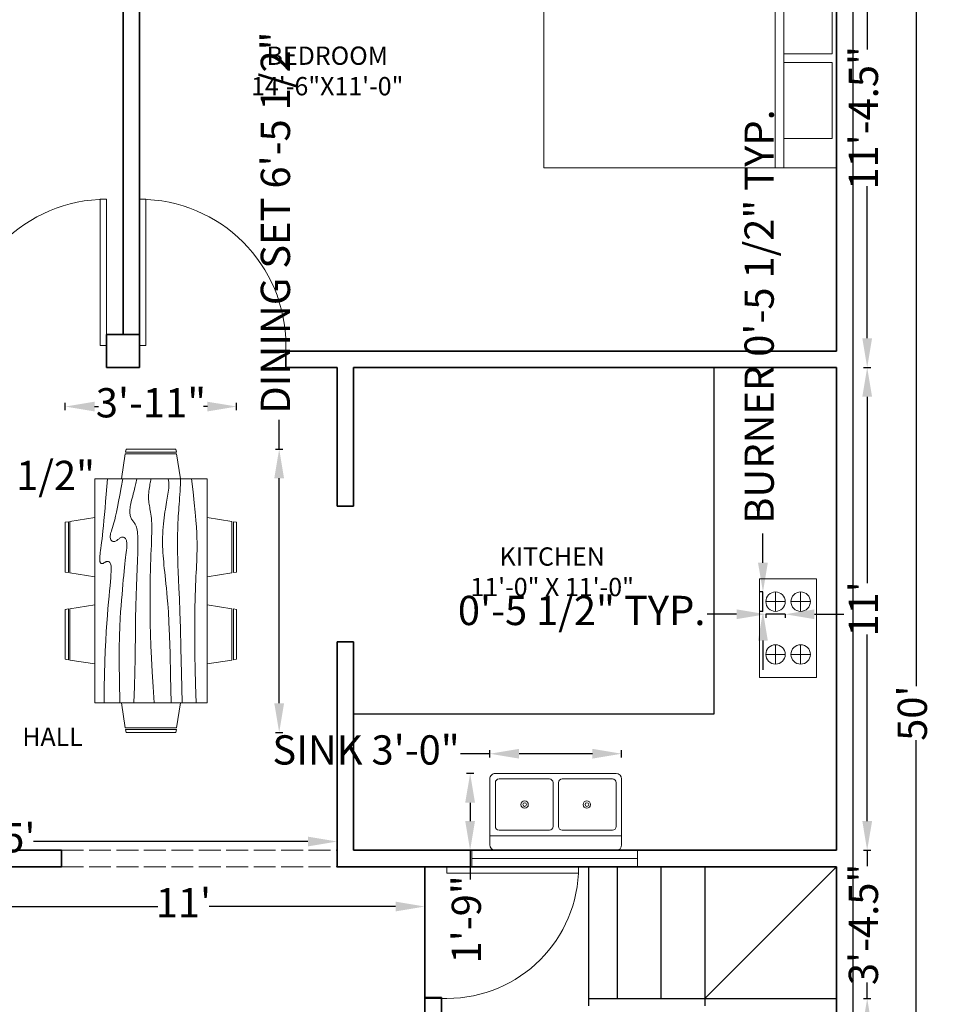
# Model space of a CAD drawing. Units: inches. Extents: x 2174 to 2692, y 577 to 1264.
# Tile 4 of 5: x 2442 to 2692, y 841 to 1110. Entities that reach past the tile are written whole.
import ezdxf

# ---------------------------------------------------------------- set-up
doc = ezdxf.new("R2010")
doc.units = ezdxf.units.IN
doc.linetypes.add('ACAD_ISO02W100', pattern=[15, 12, -3])
for name, color, linetype, lineweight in [('A-ANNO-DIMS', 2, 'Continuous', 13), ('A-AREA-IDEN', 7, 'Continuous', 18), ('A-COLS', 7, 'Continuous', 35), ('A-DOOR', 3, 'Continuous', 18), ('A-EQPM', 8, 'Continuous', 18), ('A-FLOR-CASE', 8, 'Continuous', 25), ('A-FLOR-FIXT', 9, 'Continuous', 18), ('A-FLOR-STRS', 7, 'Continuous', 25), ('A-FURN', 8, 'Continuous', 18), ('A-GLAZ', 4, 'Continuous', 18), ('A-WALL', 7, 'Continuous', 35), ('A-WALL-OVHD', 8, 'ACAD_ISO02W100', 18), ('C-PROP', 7, 'Continuous', 25)]:
    doc.layers.add(name, color=color, linetype=linetype, lineweight=lineweight)
doc.styles.get("Standard").update_dxf_attribs({"font": 'arial.ttf'})
doc.dimstyles.new('ISO-25', dxfattribs={"dimtxt": 8, "dimasz": 8, "dimexe": 1, "dimexo": 1, "dimtad": 0, "dimdec": 1, "dimlunit": 3, "dimtxsty": 'Standard', "dimcen": 2.5, "dimclrd": 1, "dimclre": 1, "dimclrt": 1, "dimadec": 0, "dimazin": 0, "dimtfac": 1, "dimtdec": 1, "dimtmove": 0, "dimatfit": 3, "dimfxl": 1, "dimfxlon": 1, "dimarcsym": 0})

# ---------------------------------------------------------------- blocks, each defined once
blk = doc.blocks.new('Dining Set - 36 x 72 in.')
for p, q in [((-22.2343, 26.00059), (-23.4847, 17.99762)), ((-22.2304, 26), (-5.7608, 26)), ((-22, 27.5), (-22.1562, 26.50042)), ((-5.8416, 26.5), (-22.1534, 26.5)), ((-22, 27.5), (-6, 27.5)), ((-5.8437, 26.49966), (-6, 27.5)), ((-4.5152, 17.99762), (-5.7655, 25.99926)), ((5.7657, 26.00059), (4.5153, 17.99762)), ((5.7696, 26), (22.2392, 26)), ((6, 27.5), (5.8438, 26.50042)), ((22.1584, 26.5), (5.8466, 26.5)), ((6, 27.5), (22, 27.5)), ((22.1563, 26.49966), (22, 27.5)), ((23.4848, 17.99762), (22.2345, 25.99926)), ((36, 18), (-36, 18)), ((-36, 18), (-36, -18)), ((36, -18), (36, 18)), ((-44.0006, 8.23428), (-35.9976, 9.48474)), ((44.0006, 8.23428), (35.9976, 9.48474)), ((-45.5, 8), (-44.5004, 8.15617)), ((-45.5, 8), (-45.5, -8)), ((-44.5, -8.15843), (-44.5, 8.15338)), ((-44, 8.23041), (-44, -8.23915)), ((44, 8.23041), (44, -8.23915)), ((44.5, -8.15843), (44.5, 8.15338)), ((45.5, 8), (44.5005, 8.15617)), ((45.5, 8), (45.5, -8)), ((-44.4997, -8.15631), (-45.5, -8)), ((-35.9976, -9.48476), (-43.9993, -8.2345)), ((35.9976, -9.48476), (43.9993, -8.2345)), ((44.4997, -8.15631), (45.5, -8)), ((-36, -18), (36, -18)), ((-22.2343, -26.0006), (-23.4847, -17.99762)), ((-4.5152, -17.99762), (-5.7655, -25.99928)), ((5.7657, -26.0006), (4.5153, -17.99762)), ((23.4848, -17.99762), (22.2345, -25.99928)), ((-22.2304, -26), (-5.7608, -26)), ((-22, -27.5), (-22.1562, -26.50044)), ((-5.8416, -26.5), (-22.1534, -26.5)), ((-22, -27.5), (-6, -27.5)), ((-5.8437, -26.49967), (-6, -27.5)), ((5.7696, -26), (22.2392, -26)), ((6, -27.5), (5.8438, -26.50044)), ((22.1584, -26.5), (5.8466, -26.5)), ((6, -27.5), (22, -27.5)), ((22.1563, -26.49967), (22, -27.5))]:
    blk.add_line(p, q)
for points in [[(-36, 15), (-31.1772, 14.97754), (-26.8079, 14.91406), (-22.8538, 14.81543), (-19.276, 14.6875), (-16.0362, 14.53613), (-13.0957, 14.36718), (-10.4159, 14.18652), (-7.9583, 14), (-5.6904, 13.81315), (-3.6035, 13.63021), (-1.6954, 13.45508), (0.0365, 13.29166), (1.5945, 13.14388), (2.9811, 13.01562), (4.1988, 12.9108), (5.25, 12.83333), (6.1393, 12.78613), (6.8802, 12.76823), (7.4883, 12.77767), (7.9792, 12.8125), (8.3685, 12.87077), (8.6719, 12.95052), (8.9049, 13.0498), (9.0833, 13.16666), (9.2205, 13.29899), (9.3216, 13.44401), (9.3895, 13.59879), (9.4271, 13.76041), (9.4373, 13.92594), (9.4232, 14.09245), (9.3875, 14.257), (9.3333, 14.41666), (9.2638, 14.56917), (9.1836, 14.71484), (9.0975, 14.85465), (9.0104, 14.98958), (8.9272, 15.1206), (8.8529, 15.2487), (8.7922, 15.37483), (8.75, 15.5), (8.7305, 15.62467), (8.7344, 15.74739), (8.7617, 15.86621), (8.8125, 15.97916), (8.8867, 16.08431), (8.9844, 16.17968), (9.1055, 16.26334), (9.25, 16.33333), (9.4189, 16.38802), (9.6172, 16.42708), (9.8506, 16.45052), (10.125, 16.45833), (10.4463, 16.45052), (10.8203, 16.42708), (11.2529, 16.38802), (11.75, 16.33333), (12.3184, 16.26318), (12.9694, 16.17838), (13.7151, 16.07991), (14.5677, 15.96875), (15.5395, 15.84586), (16.6426, 15.71224), (17.8893, 15.56884), (19.2917, 15.41666), (20.859, 15.25667), (22.5879, 15.08984), (24.4721, 14.91715), (26.5052, 14.73958), (28.6809, 14.5581), (30.9929, 14.3737), (33.4347, 14.18733), (36, 14)], [(-36, 10), (-28.9766, 10.14274), (-23.1725, 10.20442), (-18.4241, 10.19775), (-14.5677, 10.13541), (-11.4399, 10.03011), (-8.877, 9.89453), (-6.7154, 9.74137), (-4.7917, 9.58333), (-2.9698, 9.43082), (-1.2246, 9.28515), (0.4415, 9.14534), (2.026, 9.01041), (3.5266, 8.87939), (4.9408, 8.7513), (6.266, 8.62516), (7.5, 8.5), (8.6411, 8.37549), (9.6914, 8.2539), (10.6538, 8.13818), (11.5312, 8.03125), (12.3267, 7.93603), (13.043, 7.85547), (13.6831, 7.79248), (14.25, 7.75), (14.7471, 7.7303), (15.1797, 7.73307), (15.5537, 7.75732), (15.875, 7.80208), (16.1494, 7.86637), (16.3828, 7.94922), (16.5811, 8.04964), (16.75, 8.16666), (16.8944, 8.29915), (17.0143, 8.44531), (17.1089, 8.60319), (17.1771, 8.77083), (17.218, 8.94629), (17.2305, 9.1276), (17.2137, 9.31282), (17.1667, 9.5), (17.0895, 9.6875), (16.987, 9.875), (16.8649, 10.0625), (16.7292, 10.25), (16.5856, 10.4375), (16.4401, 10.625), (16.2985, 10.8125), (16.1667, 11), (16.05, 11.18733), (15.9518, 11.3737), (15.8752, 11.5581), (15.8229, 11.73958), (15.798, 11.91715), (15.8034, 12.08984), (15.842, 12.25667), (15.9167, 12.41666), (16.0295, 12.56836), (16.1784, 12.70833), (16.3605, 12.83268), (16.5729, 12.9375), (16.8127, 13.01888), (17.0768, 13.07291), (17.3625, 13.0957), (17.6667, 13.08333), (17.9894, 13.03312), (18.3418, 12.94726), (18.7382, 12.82918), (19.1927, 12.68229), (19.7195, 12.51001), (20.3327, 12.31575), (21.0465, 12.10294), (21.875, 11.875), (22.8357, 11.63354), (23.959, 11.37304), (25.2786, 11.08618), (26.8282, 10.76562), (28.6414, 10.40405), (30.752, 9.99414), (33.1936, 9.52856), (36, 9)], [(-36, 5.5), (-30.7157, 5.3348), (-26.069, 5.20963), (-21.9946, 5.11767), (-18.4271, 5.05208), (-15.3009, 5.00602), (-12.5508, 4.97265), (-10.1112, 4.94515), (-7.9167, 4.91666), (-5.909, 4.88167), (-4.0586, 4.83984), (-2.3429, 4.79215), (-0.7396, 4.73958), (0.7739, 4.6831), (2.22, 4.6237), (3.6213, 4.56233), (5, 4.5), (6.373, 4.43782), (7.7344, 4.3776), (9.0723, 4.32129), (10.375, 4.27083), (11.6309, 4.22819), (12.8281, 4.19531), (13.9551, 4.17415), (15, 4.16666), (15.954, 4.17448), (16.819, 4.19791), (17.6001, 4.23698), (18.3021, 4.29166), (18.9299, 4.36198), (19.4883, 4.44791), (19.9823, 4.54948), (20.4167, 4.66666), (20.7969, 4.79899), (21.1302, 4.94401), (21.4245, 5.09879), (21.6875, 5.26041), (21.9271, 5.42594), (22.1511, 5.59245), (22.3672, 5.757), (22.5834, 5.91666), (22.8065, 6.06868), (23.0404, 6.21093), (23.2879, 6.34147), (23.5521, 6.45833), (23.8358, 6.55957), (24.142, 6.64323), (24.4735, 6.70735), (24.8334, 6.75), (25.2235, 6.76969), (25.642, 6.76692), (26.0858, 6.74267), (26.5521, 6.69791), (27.0379, 6.63362), (27.5404, 6.55078), (28.0565, 6.45036), (28.5834, 6.33333), (29.1242, 6.19987), (29.7071, 6.04687), (30.3661, 5.87044), (31.1354, 5.66666), (32.0493, 5.43164), (33.142, 5.16146), (34.4475, 4.85221), (36, 4.5)], [(-36, -1), (-30.7915, -0.6591), (-26.0195, -0.38216), (-21.6519, -0.16284), (-17.6563, 0.00521), (-14.0005, 0.12833), (-10.6523, 0.21289), (-7.5796, 0.26522), (-4.75, 0.29166), (-2.134, 0.29793), (0.2878, 0.28711), (2.5317, 0.26163), (4.6146, 0.22396), (6.5529, 0.17651), (8.3633, 0.12174), (10.0623, 0.06209), (11.6667, 0), (13.1899, -0.06201), (14.6341, -0.1211), (15.9982, -0.17432), (17.2813, -0.21875), (18.4823, -0.25147), (19.6003, -0.26953), (20.6343, -0.27002), (21.5834, -0.25), (22.4481, -0.20768), (23.2357, -0.14584), (23.9549, -0.06836), (24.6146, 0.02083), (25.2235, 0.11784), (25.7904, 0.21875), (26.3241, 0.31966), (26.8334, 0.41666), (27.3265, 0.50618), (27.8099, 0.58593), (28.2894, 0.65397), (28.7709, 0.70833), (29.2601, 0.74707), (29.763, 0.76823), (30.2855, 0.76985), (30.8334, 0.75), (31.4088, 0.70784), (31.9994, 0.64713), (32.589, 0.57275), (33.1615, 0.48958), (33.7008, 0.4025), (34.1908, 0.3164), (34.6153, 0.23616), (34.9584, 0.16666), (35.2099, 0.11165), (35.3848, 0.07031), (35.504, 0.04069), (35.5886, 0.02083), (35.6594, 0.00879), (35.7377, 0.0026), (35.8442, 0.00032), (36, 0)], [(-36, -6.5), (-27.1843, -6.31267), (-20.084, -6.1263), (-14.469, -5.9419), (-10.1094, -5.76042), (-6.7752, -5.58285), (-4.2363, -5.41016), (-2.2629, -5.24333), (-0.625, -5.08334), (0.8708, -4.93099), (2.2715, -4.78646), (3.5872, -4.64974), (4.8281, -4.52084), (6.0046, -4.39974), (7.127, -4.28646), (8.2053, -4.18099), (9.25, -4.08334), (10.2705, -3.99382), (11.2734, -3.91407), (12.2647, -3.84603), (13.25, -3.79167), (14.2354, -3.75293), (15.2266, -3.73177), (16.2295, -3.73015), (17.25, -3.75), (18.2912, -3.79248), (19.3451, -3.85547), (20.4009, -3.93604), (21.4479, -4.03125), (22.4754, -4.13819), (23.4727, -4.25391), (24.4289, -4.37549), (25.3334, -4.5), (26.1785, -4.62492), (26.9694, -4.74935), (27.7145, -4.87281), (28.4219, -4.99479), (29.1, -5.11483), (29.7572, -5.23242), (30.4016, -5.34709), (31.0417, -5.45834), (31.6837, -5.56437), (32.3262, -5.65821), (32.9658, -5.73153), (33.599, -5.77604), (34.2224, -5.78345), (34.8327, -5.74545), (35.4264, -5.65373), (36, -5.5)], [(-36, -10), (-26.4022, -9.81299), (-18.4675, -9.62891), (-11.9839, -9.45069), (-6.7396, -9.28125), (-2.5226, -9.12354), (0.8789, -8.98047), (3.6769, -8.85498), (6.0833, -8.75), (8.2767, -8.66765), (10.3021, -8.60677), (12.1712, -8.56543), (13.8958, -8.54167), (15.4876, -8.53353), (16.9583, -8.53907), (18.3197, -8.55632), (19.5834, -8.58334), (20.7616, -8.61841), (21.8685, -8.66081), (22.9188, -8.71004), (23.9271, -8.76563), (24.9081, -8.82707), (25.8763, -8.89388), (26.8465, -8.96558), (27.8334, -9.04167), (28.8474, -9.12118), (29.8828, -9.20117), (30.93, -9.27824), (31.9792, -9.34896), (33.0205, -9.40991), (34.0443, -9.45768), (35.0407, -9.48885), (36, -9.5)], [(-36, -14.5), (-30.0881, -14.33513), (-25.0332, -14.21224), (-20.7312, -14.12647), (-17.0781, -14.07292), (-13.97, -14.04671), (-11.3027, -14.04297), (-8.9724, -14.05681), (-6.875, -14.08334), (-4.9224, -14.11833), (-3.0905, -14.16016), (-1.3709, -14.20785), (0.2448, -14.26042), (1.7647, -14.3169), (3.1973, -14.3763), (4.5507, -14.43767), (5.8333, -14.5), (7.0554, -14.5621), (8.235, -14.62175), (9.3922, -14.67652), (10.5469, -14.72396), (11.7192, -14.76164), (12.929, -14.78711), (14.1965, -14.79794), (15.5417, -14.79167), (16.9933, -14.76424), (18.6152, -14.70508), (20.4804, -14.60197), (22.6615, -14.44271), (25.2312, -14.21509), (28.2624, -13.9069), (31.8277, -13.50594), (36, -13)]]:
    blk.add_lwpolyline(points)
blk = doc.blocks.new('Sink-double - 36 in top')
for p, q in [((-18, -4), (18, -4)), ((-0.75, -18.5), (-0.75, -6.5)), ((0.75, -6.5), (0.75, -18.5))]:
    blk.add_line(p, q)
for points in [[(-16.5, 0), (16.5, 0)], [(-18, -19.5), (-18, -1.5)], [(18, -1.5), (18, -19.5)], [(-16.5, -18.5), (-16.5, -6.5)], [(-15.5, -5.5), (-1.75, -5.5)], [(1.75, -5.5), (15.5, -5.5)], [(16.5, -6.5), (16.5, -18.5)], [(16.5, -21), (-16.5, -21)], [(-1.75, -19.5), (-15.5, -19.5)], [(15.5, -19.5), (1.75, -19.5)]]:
    blk.add_lwpolyline(points)
for centre, radius in [((-8.5, -12.5), 1), ((-8.5, -12.5), 0.5), ((8.5, -12.5), 1), ((8.5, -12.5), 0.5)]:
    blk.add_circle(centre, radius)
for centre, radius, start, end in [((-16.5, -1.5), 1.5, 90, 180), ((16.5, -1.5), 1.5, 0, 90), ((-15.5, -6.5), 1, 90, 180), ((-1.75, -6.5), 1, 0, 90), ((1.75, -6.5), 1, 90, 180), ((15.5, -6.5), 1, 0, 90), ((-15.5, -18.5), 1, 180, 270), ((-1.75, -18.5), 1, 270, 0), ((1.75, -18.5), 1, 180, 270), ((15.5, -18.5), 1, 270, 0), ((-16.5, -19.5), 1.5, 180, 270), ((16.5, -19.5), 1.5, 270, 0)]:
    blk.add_arc(centre, radius, start, end)
blk = doc.blocks.new('Bed - Queen')
for p, q in [((0, -80.00003), (0, 0)), ((0, 0), (59.99999, 0)), ((59.99999, 0), (59.99999, -80.00003)), ((7.99999, -1.2), (28.79998, -1.2)), ((7.99999, -14.4), (7.99999, -1.2)), ((28.79998, -1.2), (28.79998, -14.4)), ((31.19999, -1.2), (51.99999, -1.2)), ((31.19999, -14.4), (31.19999, -1.2)), ((51.99999, -1.2), (51.99999, -16.4)), ((0, -14.4), (44.8, -14.4)), ((59.99999, -29.6), (44.8, -14.4)), ((44.8, -14.4), (44.8, -29.6)), ((44.8, -16.8), (0, -16.8)), ((51.99999, -16.4), (46.79936, -16.4)), ((44.8, -29.6), (59.99999, -29.6)), ((59.99999, -80.00003), (0, -80.00003))]:
    blk.add_line(p, q)
blk = doc.blocks.new('*D12')
at = {"layer": 'A-ANNO-DIMS', "color": 0, "lineweight": -2, "transparency": 16777216}
for p, q in [((2348.95, 885.56), (2348.95, 884.25)), ((2356.95, 885.25), (2431.92, 885.25)), ((2520.95, 885.25), (2445.99, 885.25)), ((2528.95, 885.56), (2528.95, 884.25))]:
    blk.add_line(p, q, dxfattribs=at)
at = {"layer": 'A-ANNO-DIMS', "color": 0, "transparency": 16777216}
for points in [[(2356.95, 886.58), (2356.95, 883.91), (2348.95, 885.25)], [(2520.95, 886.58), (2520.95, 883.91), (2528.95, 885.25)]]:
    blk.add_solid(points, dxfattribs=at)
at = {"layer": 'Defpoints', "color": 0, "transparency": 16777216}
for p in [(2348.95, 886.56), (2528.95, 886.56), (2348.95, 885.25)]:
    blk.add_point(p, dxfattribs=at)
at = {"layer": 'A-ANNO-DIMS', "color": 0, "transparency": 16777216, "insert": (2438.95, 885.25), "char_height": 8, "attachment_point": 5}
blk.add_mtext("15'", dxfattribs=at)
blk = doc.blocks.new('*D13')
at = {"layer": 'A-ANNO-DIMS', "color": 0, "lineweight": -2, "transparency": 16777216}
for p, q in [((2420.95, 868.48), (2420.95, 866.48)), ((2428.95, 867.48), (2479.92, 867.48)), ((2544.95, 867.48), (2493.99, 867.48)), ((2552.95, 868.48), (2552.95, 866.48))]:
    blk.add_line(p, q, dxfattribs=at)
at = {"layer": 'A-ANNO-DIMS', "color": 0, "transparency": 16777216}
for points in [[(2428.95, 868.81), (2428.95, 866.15), (2420.95, 867.48)], [(2544.95, 868.81), (2544.95, 866.15), (2552.95, 867.48)]]:
    blk.add_solid(points, dxfattribs=at)
at = {"layer": 'Defpoints', "color": 0, "transparency": 16777216}
for p in [(2420.95, 878.35), (2552.95, 878.35), (2420.95, 867.48)]:
    blk.add_point(p, dxfattribs=at)
at = {"layer": 'A-ANNO-DIMS', "color": 0, "transparency": 16777216, "insert": (2486.95, 867.48), "char_height": 8, "attachment_point": 5}
blk.add_mtext("11'", dxfattribs=at)
blk = doc.blocks.new('*U27')
for p, q in [((0, 0), (0, -6)), ((36, 0), (36, -6))]:
    blk.add_line(p, q)
blk.add_lwpolyline([(0, 0), (0, 36), (1.75, 36), (1.75, 0)], close=True)
blk.add_arc((0, 0), 36, 0, 90)
blk = doc.blocks.new('*U20')
for p, q in [((0, 0), (0, -6)), ((40, 0), (40, -6))]:
    blk.add_line(p, q)
blk.add_lwpolyline([(0, 0), (0, 40), (1.75, 40), (1.75, 0)], close=True)
blk.add_arc((0, 0), 40, 0, 90)
blk = doc.blocks.new('*U24')
for p, q in [((0, 0), (0, -6)), ((-40, 0), (-40, -6))]:
    blk.add_line(p, q)
blk.add_lwpolyline([(0, 0), (0, 40), (-1.75, 40), (-1.75, 0)], close=True)
blk.add_arc((0, 0), 40, 90, 180)
blk = doc.blocks.new('*D36')
at = {"layer": 'A-ANNO-DIMS', "color": 0, "lineweight": -2, "transparency": 16777216}
for p, q in [((2672.81, 1151.35), (2674.81, 1151.35)), ((2673.81, 1143.35), (2673.81, 1101.75)), ((2673.81, 1022.85), (2673.81, 1064.45)), ((2672.81, 1014.85), (2674.81, 1014.85))]:
    blk.add_line(p, q, dxfattribs=at)
at = {"layer": 'A-ANNO-DIMS', "color": 0, "transparency": 16777216}
for points in [[(2672.48, 1143.35), (2675.15, 1143.35), (2673.81, 1151.35)], [(2672.48, 1022.85), (2675.15, 1022.85), (2673.81, 1014.85)]]:
    blk.add_solid(points, dxfattribs=at)
at = {"layer": 'Defpoints', "color": 0, "transparency": 16777216}
for p in [(2665.45, 1151.35), (2665.45, 1014.85), (2673.81, 1014.85)]:
    blk.add_point(p, dxfattribs=at)
at = {"layer": 'A-ANNO-DIMS', "color": 0, "transparency": 16777216, "insert": (2673.81, 1083.1), "char_height": 8, "attachment_point": 5, "rotation": 90}
blk.add_mtext('11\'-4.5"', dxfattribs=at)
blk = doc.blocks.new('*D37')
at = {"layer": 'A-ANNO-DIMS', "color": 0, "lineweight": -2, "transparency": 16777216}
for p, q in [((2672.81, 1014.85), (2674.81, 1014.85)), ((2673.81, 1006.85), (2673.81, 955.89)), ((2673.81, 890.85), (2673.81, 941.81)), ((2672.81, 882.85), (2674.81, 882.85))]:
    blk.add_line(p, q, dxfattribs=at)
at = {"layer": 'A-ANNO-DIMS', "color": 0, "transparency": 16777216}
for points in [[(2672.48, 1006.85), (2675.15, 1006.85), (2673.81, 1014.85)], [(2672.48, 890.85), (2675.15, 890.85), (2673.81, 882.85)]]:
    blk.add_solid(points, dxfattribs=at)
at = {"layer": 'Defpoints', "color": 0, "transparency": 16777216}
for p in [(2665.45, 1014.85), (2665.45, 882.85), (2673.81, 882.85)]:
    blk.add_point(p, dxfattribs=at)
at = {"layer": 'A-ANNO-DIMS', "color": 0, "transparency": 16777216, "insert": (2673.81, 948.85), "char_height": 8, "attachment_point": 5, "rotation": 90}
blk.add_mtext("11'", dxfattribs=at)
blk = doc.blocks.new('*D38')
at = {"layer": 'A-ANNO-DIMS', "color": 0, "lineweight": -2, "transparency": 16777216}
for p, q in [((2673.81, 890.85), (2673.81, 898.85)), ((2672.81, 882.85), (2674.81, 882.85)), ((2673.81, 882.85), (2673.81, 878.52)), ((2673.81, 842.35), (2673.81, 846.69)), ((2672.81, 842.35), (2674.81, 842.35)), ((2673.81, 834.35), (2673.81, 826.35))]:
    blk.add_line(p, q, dxfattribs=at)
at = {"layer": 'A-ANNO-DIMS', "color": 0, "transparency": 16777216}
for points in [[(2672.48, 890.85), (2675.15, 890.85), (2673.81, 882.85)], [(2672.48, 834.35), (2675.15, 834.35), (2673.81, 842.35)]]:
    blk.add_solid(points, dxfattribs=at)
at = {"layer": 'Defpoints', "color": 0, "transparency": 16777216}
for p in [(2665.45, 882.85), (2665.45, 842.35), (2673.81, 842.35)]:
    blk.add_point(p, dxfattribs=at)
at = {"layer": 'A-ANNO-DIMS', "color": 0, "transparency": 16777216, "insert": (2673.81, 862.6), "char_height": 8, "attachment_point": 5, "rotation": 90}
blk.add_mtext('3\'-4.5"', dxfattribs=at)
blk = doc.blocks.new('*D39')
at = {"layer": 'A-ANNO-DIMS', "color": 0, "lineweight": -2, "transparency": 16777216}
for p, q in [((2672.81, 842.35), (2674.81, 842.35)), ((2673.81, 834.35), (2673.81, 810.68)), ((2673.81, 778.35), (2673.81, 802.02)), ((2672.81, 770.35), (2674.81, 770.35))]:
    blk.add_line(p, q, dxfattribs=at)
at = {"layer": 'A-ANNO-DIMS', "color": 0, "transparency": 16777216}
for points in [[(2672.48, 834.35), (2675.15, 834.35), (2673.81, 842.35)], [(2672.48, 778.35), (2675.15, 778.35), (2673.81, 770.35)]]:
    blk.add_solid(points, dxfattribs=at)
at = {"layer": 'Defpoints', "color": 0, "transparency": 16777216}
for p in [(2665.45, 842.35), (2665.45, 770.35), (2673.81, 770.35)]:
    blk.add_point(p, dxfattribs=at)
at = {"layer": 'A-ANNO-DIMS', "color": 0, "transparency": 16777216, "insert": (2673.81, 806.35), "char_height": 8, "attachment_point": 5, "rotation": 90}
blk.add_mtext("6'", dxfattribs=at)
blk = doc.blocks.new('*D42')
at = {"layer": 'A-ANNO-DIMS', "color": 0, "lineweight": -2, "transparency": 16777216}
for p, q in [((2686.18, 1220.35), (2688.18, 1220.35)), ((2687.18, 1212.35), (2687.18, 927.77)), ((2687.18, 628.35), (2687.18, 912.94)), ((2686.18, 620.35), (2688.18, 620.35))]:
    blk.add_line(p, q, dxfattribs=at)
at = {"layer": 'A-ANNO-DIMS', "color": 0, "transparency": 16777216}
for points in [[(2685.84, 1212.35), (2688.51, 1212.35), (2687.18, 1220.35)], [(2685.84, 628.35), (2688.51, 628.35), (2687.18, 620.35)]]:
    blk.add_solid(points, dxfattribs=at)
at = {"layer": 'Defpoints', "color": 0, "transparency": 16777216}
for p in [(2669.95, 1220.35), (2687.18, 1220.35), (2669.95, 620.35)]:
    blk.add_point(p, dxfattribs=at)
at = {"layer": 'A-ANNO-DIMS', "color": 0, "transparency": 16777216, "insert": (2687.18, 920.35), "char_height": 8, "attachment_point": 5, "rotation": 90}
blk.add_mtext("50'", dxfattribs=at)
blk = doc.blocks.new('COOKTOP-BURNER')
for p, q in [((2.65, 0), (-2.65, 0)), ((0, -2.65), (0, 2.65))]:
    blk.add_line(p, q)
blk.add_circle((0, 0), 2.65)
blk = doc.blocks.new('*D49')
at = {"layer": 'A-ANNO-DIMS', "color": 1, "lineweight": -2, "transparency": 16777216}
for p, q in [((2645.32, 961.48), (2645.32, 969.48)), ((2645.32, 953.48), (2644.32, 953.48)), ((2645.32, 948.18), (2645.32, 953.48)), ((2645.32, 948.18), (2644.32, 948.18)), ((2645.32, 940.18), (2645.32, 932.18))]:
    blk.add_line(p, q, dxfattribs=at)
at = {"layer": 'A-ANNO-DIMS', "color": 1, "transparency": 16777216}
for points in [[(2643.98, 961.48), (2646.65, 961.48), (2645.32, 953.48)], [(2643.98, 940.18), (2646.65, 940.18), (2645.32, 948.18)]]:
    blk.add_solid(points, dxfattribs=at)
at = {"layer": 'Defpoints', "color": 0, "transparency": 16777216}
for p in [(2645.32, 953.48), (2646.11, 953.48), (2646.11, 948.18)]:
    blk.add_point(p, dxfattribs=at)
at = {"layer": 'A-ANNO-DIMS', "color": 1, "transparency": 16777216, "insert": (2645.32, 1028.78), "char_height": 8, "attachment_point": 5, "rotation": 90}
blk.add_mtext('BURNER 0\'-5 1/2" TYP.', dxfattribs=at)
blk = doc.blocks.new('*D50')
at = {"layer": 'A-ANNO-DIMS', "color": 1, "lineweight": -2, "transparency": 16777216}
for p, q in [((2638.11, 947.39), (2630.11, 947.39)), ((2646.11, 947.39), (2646.11, 946.39)), ((2651.41, 947.39), (2646.11, 947.39)), ((2651.41, 947.39), (2651.41, 946.39)), ((2659.41, 947.39), (2667.41, 947.39))]:
    blk.add_line(p, q, dxfattribs=at)
at = {"layer": 'A-ANNO-DIMS', "color": 1, "transparency": 16777216}
for points in [[(2638.11, 948.72), (2638.11, 946.05), (2646.11, 947.39)], [(2659.41, 948.72), (2659.41, 946.05), (2651.41, 947.39)]]:
    blk.add_solid(points, dxfattribs=at)
at = {"layer": 'Defpoints', "color": 0, "transparency": 16777216}
for p in [(2646.11, 948.18), (2651.41, 948.18), (2646.11, 947.39)]:
    blk.add_point(p, dxfattribs=at)
at = {"layer": 'A-ANNO-DIMS', "color": 1, "transparency": 16777216, "insert": (2595.78, 947.39), "char_height": 8, "attachment_point": 5}
blk.add_mtext('0\'-5 1/2" TYP.', dxfattribs=at)
blk = doc.blocks.new('*D54')
at = {"layer": 'A-ANNO-DIMS', "color": 1, "lineweight": -2, "transparency": 16777216}
for p, q in [((2388.24, 985.3), (2388.24, 983.3)), ((2412.67, 985.3), (2412.67, 983.3)), ((2396.24, 984.3), (2404.67, 984.3)), ((2412.67, 984.3), (2420.67, 984.3))]:
    blk.add_line(p, q, dxfattribs=at)
at = {"layer": 'A-ANNO-DIMS', "color": 1, "transparency": 16777216}
for points in [[(2396.24, 985.64), (2396.24, 982.97), (2388.24, 984.3)], [(2404.67, 985.64), (2404.67, 982.97), (2412.67, 984.3)]]:
    blk.add_solid(points, dxfattribs=at)
at = {"layer": 'Defpoints', "color": 0, "transparency": 16777216}
for p in [(2388.24, 988.35), (2412.67, 988.35), (2412.67, 984.3)]:
    blk.add_point(p, dxfattribs=at)
at = {"layer": 'A-ANNO-DIMS', "color": 1, "transparency": 16777216, "insert": (2441.32, 984.3), "char_height": 8, "attachment_point": 5}
blk.add_mtext('2\'-0 1/2"', dxfattribs=at)
blk = doc.blocks.new('*D55')
at = {"layer": 'A-ANNO-DIMS', "color": 1, "lineweight": -2, "transparency": 16777216}
for p, q in [((2513.12, 992.55), (2513.12, 1000.55)), ((2512.12, 992.55), (2514.12, 992.55)), ((2513.12, 923.06), (2513.12, 984.55)), ((2512.12, 915.06), (2514.12, 915.06))]:
    blk.add_line(p, q, dxfattribs=at)
at = {"layer": 'A-ANNO-DIMS', "color": 1, "transparency": 16777216}
for points in [[(2511.78, 984.55), (2514.45, 984.55), (2513.12, 992.55)], [(2511.78, 923.06), (2514.45, 923.06), (2513.12, 915.06)]]:
    blk.add_solid(points, dxfattribs=at)
at = {"layer": 'Defpoints', "color": 0, "transparency": 16777216}
for p in [(2501.49, 992.55), (2513.12, 992.55), (2501.49, 915.06)]:
    blk.add_point(p, dxfattribs=at)
at = {"layer": 'A-ANNO-DIMS', "color": 1, "transparency": 16777216, "insert": (2513.12, 1054.46), "char_height": 8, "attachment_point": 5, "rotation": 90}
blk.add_mtext('DINING SET 6\'-5 1/2"', dxfattribs=at)
blk = doc.blocks.new('*D56')
at = {"layer": 'A-ANNO-DIMS', "color": 1, "lineweight": -2, "transparency": 16777216}
for p, q in [((2454.66, 1003.17), (2454.66, 1005.17)), ((2462.66, 1004.17), (2463.71, 1004.17)), ((2493.49, 1004.17), (2492.44, 1004.17)), ((2501.49, 1003.17), (2501.49, 1005.17))]:
    blk.add_line(p, q, dxfattribs=at)
at = {"layer": 'A-ANNO-DIMS', "color": 1, "transparency": 16777216}
for points in [[(2462.66, 1005.5), (2462.66, 1002.84), (2454.66, 1004.17)], [(2493.49, 1005.5), (2493.49, 1002.84), (2501.49, 1004.17)]]:
    blk.add_solid(points, dxfattribs=at)
at = {"layer": 'Defpoints', "color": 0, "transparency": 16777216}
for p in [(2454.66, 1004.17), (2454.66, 992.55), (2501.49, 992.55)]:
    blk.add_point(p, dxfattribs=at)
at = {"layer": 'A-ANNO-DIMS', "color": 1, "transparency": 16777216, "insert": (2478.08, 1004.17), "char_height": 8, "attachment_point": 5}
blk.add_mtext('3\'-11"', dxfattribs=at)
blk = doc.blocks.new('*D59')
at = {"layer": 'A-ANNO-DIMS', "color": 1, "lineweight": -2, "transparency": 16777216}
for p, q in [((2570.7, 908.25), (2570.7, 910.25)), ((2606.7, 908.25), (2606.7, 910.25)), ((2570.7, 909.25), (2562.7, 909.25)), ((2598.7, 909.25), (2578.7, 909.25))]:
    blk.add_line(p, q, dxfattribs=at)
at = {"layer": 'A-ANNO-DIMS', "color": 1, "transparency": 16777216}
for points in [[(2578.7, 910.59), (2578.7, 907.92), (2570.7, 909.25)], [(2598.7, 910.59), (2598.7, 907.92), (2606.7, 909.25)]]:
    blk.add_solid(points, dxfattribs=at)
at = {"layer": 'Defpoints', "color": 0, "transparency": 16777216}
for p in [(2570.7, 909.25), (2570.7, 903.85), (2606.7, 903.85)]:
    blk.add_point(p, dxfattribs=at)
at = {"layer": 'A-ANNO-DIMS', "color": 1, "transparency": 16777216, "insert": (2536.86, 909.25), "char_height": 8, "attachment_point": 5}
blk.add_mtext('SINK 3\'-0"', dxfattribs=at)
blk = doc.blocks.new('*D60')
at = {"layer": 'A-ANNO-DIMS', "color": 1, "lineweight": -2, "transparency": 16777216}
for p, q in [((2566.3, 903.85), (2564.3, 903.85)), ((2565.3, 895.85), (2565.3, 890.85)), ((2566.3, 882.85), (2564.3, 882.85)), ((2565.3, 882.85), (2565.3, 874.85))]:
    blk.add_line(p, q, dxfattribs=at)
at = {"layer": 'A-ANNO-DIMS', "color": 1, "transparency": 16777216}
for points in [[(2563.96, 895.85), (2566.63, 895.85), (2565.3, 903.85)], [(2563.96, 890.85), (2566.63, 890.85), (2565.3, 882.85)]]:
    blk.add_solid(points, dxfattribs=at)
at = {"layer": 'Defpoints', "color": 0, "transparency": 16777216}
for p in [(2570.7, 903.85), (2565.3, 882.85), (2570.7, 882.85)]:
    blk.add_point(p, dxfattribs=at)
at = {"layer": 'A-ANNO-DIMS', "color": 1, "transparency": 16777216, "insert": (2565.3, 863.97), "char_height": 8, "attachment_point": 5, "rotation": 90}
blk.add_mtext('1\'-9"', dxfattribs=at)
blk = doc.blocks.new('*D64')
at = {"layer": 'A-ANNO-DIMS', "color": 1, "lineweight": -2, "transparency": 16777216}
for p, q in [((2474.95, 590.4), (2474.95, 588.4)), ((2514.95, 590.4), (2514.95, 588.4)), ((2482.95, 589.4), (2483.7, 589.4)), ((2506.95, 589.4), (2506.21, 589.4))]:
    blk.add_line(p, q, dxfattribs=at)
at = {"layer": 'A-ANNO-DIMS', "color": 1, "transparency": 16777216}
for points in [[(2482.95, 590.74), (2482.95, 588.07), (2474.95, 589.4)], [(2506.95, 590.74), (2506.95, 588.07), (2514.95, 589.4)]]:
    blk.add_solid(points, dxfattribs=at)
at = {"layer": 'Defpoints', "color": 0, "transparency": 16777216}
for p in [(2474.95, 1014.85), (2514.95, 1014.85), (2514.95, 589.4)]:
    blk.add_point(p, dxfattribs=at)
at = {"layer": 'A-ANNO-DIMS', "color": 1, "transparency": 16777216, "insert": (2494.95, 589.4), "char_height": 8, "attachment_point": 5}
blk.add_mtext('3\'-4"', dxfattribs=at)
blk = doc.blocks.new('*D65')
at = {"layer": 'A-ANNO-DIMS', "color": 1, "lineweight": -2, "transparency": 16777216}
for p, q in [((2420.95, 1250.3), (2420.95, 1252.3)), ((2454.95, 1250.3), (2454.95, 1252.3)), ((2412.95, 1251.3), (2404.95, 1251.3)), ((2420.95, 1251.3), (2423.52, 1251.3)), ((2454.95, 1251.3), (2452.39, 1251.3)), ((2462.95, 1251.3), (2470.95, 1251.3))]:
    blk.add_line(p, q, dxfattribs=at)
at = {"layer": 'A-ANNO-DIMS', "color": 1, "transparency": 16777216}
for points in [[(2412.95, 1252.64), (2412.95, 1249.97), (2420.95, 1251.3)], [(2462.95, 1252.64), (2462.95, 1249.97), (2454.95, 1251.3)]]:
    blk.add_solid(points, dxfattribs=at)
at = {"layer": 'Defpoints', "color": 0, "transparency": 16777216}
for p in [(2454.95, 1251.3), (2420.95, 698.35), (2454.95, 698.35)]:
    blk.add_point(p, dxfattribs=at)
at = {"layer": 'A-ANNO-DIMS', "color": 1, "transparency": 16777216, "insert": (2437.95, 1251.3), "char_height": 8, "attachment_point": 5}
blk.add_mtext('2\'-10"', dxfattribs=at)
blk = doc.blocks.new('*D66')
at = {"layer": 'A-ANNO-DIMS', "color": 1, "lineweight": -2, "transparency": 16777216}
for p, q in [((2454.95, 1250.3), (2454.95, 1252.3)), ((2518.95, 1250.3), (2518.95, 1252.3)), ((2462.95, 1251.3), (2475.7, 1251.3)), ((2510.95, 1251.3), (2498.21, 1251.3))]:
    blk.add_line(p, q, dxfattribs=at)
at = {"layer": 'A-ANNO-DIMS', "color": 1, "transparency": 16777216}
for points in [[(2462.95, 1252.64), (2462.95, 1249.97), (2454.95, 1251.3)], [(2510.95, 1252.64), (2510.95, 1249.97), (2518.95, 1251.3)]]:
    blk.add_solid(points, dxfattribs=at)
at = {"layer": 'Defpoints', "color": 0, "transparency": 16777216}
for p in [(2518.95, 1251.3), (2454.95, 698.35), (2518.95, 698.35)]:
    blk.add_point(p, dxfattribs=at)
at = {"layer": 'A-ANNO-DIMS', "color": 1, "transparency": 16777216, "insert": (2486.95, 1251.3), "char_height": 8, "attachment_point": 5}
blk.add_mtext('5\'-4"', dxfattribs=at)
blk = doc.blocks.new('*D69')
at = {"layer": 'A-ANNO-DIMS', "color": 1, "lineweight": -2, "transparency": 16777216}
for p, q in [((2453.65, 1250.3), (2453.65, 1252.3)), ((2528.95, 1250.3), (2528.95, 1252.3)), ((2461.65, 1251.3), (2470.7, 1251.3)), ((2520.95, 1251.3), (2511.9, 1251.3))]:
    blk.add_line(p, q, dxfattribs=at)
at = {"layer": 'A-ANNO-DIMS', "color": 1, "transparency": 16777216}
for points in [[(2461.65, 1252.64), (2461.65, 1249.97), (2453.65, 1251.3)], [(2520.95, 1252.64), (2520.95, 1249.97), (2528.95, 1251.3)]]:
    blk.add_solid(points, dxfattribs=at)
at = {"layer": 'Defpoints', "color": 0, "transparency": 16777216}
for p in [(2528.95, 1251.3), (2453.65, 878.35), (2528.95, 878.35)]:
    blk.add_point(p, dxfattribs=at)
at = {"layer": 'A-ANNO-DIMS', "color": 1, "transparency": 16777216, "insert": (2491.3, 1251.3), "char_height": 8, "attachment_point": 5}
blk.add_mtext('6\'-3 1/2"', dxfattribs=at)
blk = doc.blocks.new('*D70')
at = {"layer": 'A-ANNO-DIMS', "color": 1, "lineweight": -2, "transparency": 16777216}
for p, q in [((2261, 984.94), (2261, 992.94)), ((2262, 976.94), (2260, 976.94)), ((2261, 976.94), (2261, 969.66)), ((2261, 939.87), (2261, 947.15)), ((2262, 939.87), (2260, 939.87)), ((2261, 931.87), (2261, 923.87))]:
    blk.add_line(p, q, dxfattribs=at)
at = {"layer": 'A-ANNO-DIMS', "color": 1, "transparency": 16777216}
for points in [[(2259.67, 984.94), (2262.34, 984.94), (2261, 976.94)], [(2259.67, 931.87), (2262.34, 931.87), (2261, 939.87)]]:
    blk.add_solid(points, dxfattribs=at)
at = {"layer": 'Defpoints', "color": 0, "transparency": 16777216}
for p in [(2528.95, 976.94), (2261, 939.87), (2528.95, 939.87)]:
    blk.add_point(p, dxfattribs=at)
at = {"layer": 'A-ANNO-DIMS', "color": 1, "transparency": 16777216, "insert": (2261, 958.41), "char_height": 8, "attachment_point": 5, "rotation": 90}
blk.add_mtext('3\'-1"', dxfattribs=at)
blk = doc.blocks.new('*D74')
at = {"layer": 'A-ANNO-DIMS', "color": 1, "lineweight": -2, "transparency": 16777216}
for p, q in [((2565.76, 1250.3), (2565.76, 1252.3)), ((2611.08, 1250.3), (2611.08, 1252.3)), ((2557.76, 1251.3), (2549.76, 1251.3)), ((2565.76, 1251.3), (2567.84, 1251.3)), ((2611.08, 1251.3), (2609, 1251.3)), ((2619.08, 1251.3), (2627.08, 1251.3))]:
    blk.add_line(p, q, dxfattribs=at)
at = {"layer": 'A-ANNO-DIMS', "color": 1, "transparency": 16777216}
for points in [[(2557.76, 1252.64), (2557.76, 1249.97), (2565.76, 1251.3)], [(2619.08, 1252.64), (2619.08, 1249.97), (2611.08, 1251.3)]]:
    blk.add_solid(points, dxfattribs=at)
at = {"layer": 'Defpoints', "color": 0, "transparency": 16777216}
for p in [(2611.08, 1251.3), (2565.76, 882.85), (2611.08, 882.85)]:
    blk.add_point(p, dxfattribs=at)
at = {"layer": 'A-ANNO-DIMS', "color": 1, "transparency": 16777216, "insert": (2588.42, 1251.3), "char_height": 8, "attachment_point": 5}
blk.add_mtext('3\'-9 1/2"', dxfattribs=at)
blk = doc.blocks.new('*D78')
at = {"layer": 'A-ANNO-DIMS', "color": 1, "lineweight": -2, "transparency": 16777216}
for p, q in [((2399.49, 590.4), (2399.49, 588.4)), ((2432.76, 590.4), (2432.76, 588.4)), ((2407.49, 589.4), (2424.76, 589.4)), ((2432.76, 589.4), (2440.76, 589.4))]:
    blk.add_line(p, q, dxfattribs=at)
at = {"layer": 'A-ANNO-DIMS', "color": 1, "transparency": 16777216}
for points in [[(2407.49, 590.74), (2407.49, 588.07), (2399.49, 589.4)], [(2424.76, 590.74), (2424.76, 588.07), (2432.76, 589.4)]]:
    blk.add_solid(points, dxfattribs=at)
at = {"layer": 'Defpoints', "color": 0, "transparency": 16777216}
for p in [(2399.49, 1151.35), (2432.76, 1151.35), (2432.76, 589.4)]:
    blk.add_point(p, dxfattribs=at)
at = {"layer": 'A-ANNO-DIMS', "color": 1, "transparency": 16777216, "insert": (2461.41, 589.4), "char_height": 8, "attachment_point": 5}
blk.add_mtext('2\'-9 1/2"', dxfattribs=at)
blk = doc.blocks.new('*D80')
at = {"layer": 'A-ANNO-DIMS', "color": 1, "lineweight": -2, "transparency": 16777216}
for p, q in [((2577.45, 590.4), (2577.45, 588.4)), ((2665.45, 590.4), (2665.45, 588.4)), ((2585.45, 589.4), (2610.23, 589.4)), ((2657.45, 589.4), (2632.68, 589.4))]:
    blk.add_line(p, q, dxfattribs=at)
at = {"layer": 'A-ANNO-DIMS', "color": 1, "transparency": 16777216}
for points in [[(2585.45, 590.74), (2585.45, 588.07), (2577.45, 589.4)], [(2657.45, 590.74), (2657.45, 588.07), (2665.45, 589.4)]]:
    blk.add_solid(points, dxfattribs=at)
at = {"layer": 'Defpoints', "color": 0, "transparency": 16777216}
for p in [(2577.45, 1215.85), (2665.45, 1215.85), (2665.45, 589.4)]:
    blk.add_point(p, dxfattribs=at)
at = {"layer": 'A-ANNO-DIMS', "color": 1, "transparency": 16777216, "insert": (2621.45, 589.4), "char_height": 8, "attachment_point": 5}
blk.add_mtext('7\'-4"', dxfattribs=at)

msp = doc.modelspace()

# ---------------------------------------------------------------- linework, layer by layer
at = {"layer": 'A-COLS'}
for p, q in [((2465.95, 1014.85), (2465.95, 1023.85)), ((2465.95, 1023.85), (2474.95, 1023.85)), ((2474.95, 1019.35), (2474.95, 1014.85)), ((2474.95, 1014.85), (2465.95, 1014.85)), ((2474.95, 1014.85), (2470.45, 1014.85))]:
    msp.add_line(p, q, dxfattribs=at)
at = {"layer": 'A-EQPM'}
msp.add_lwpolyline([(2644.41, 957.11), (2659.98, 957.11), (2659.98, 930.13), (2644.41, 930.13)], close=True, dxfattribs=at)
at = {"layer": 'A-FLOR-CASE'}
for p, q in [((2631.88, 1014.85), (2631.88, 920.06)), ((2631.88, 920.06), (2533.45, 920.06))]:
    msp.add_line(p, q, dxfattribs=at)
at = {"layer": 'A-FLOR-STRS'}
for p, q in [((2597.63, 878.35), (2597.63, 840.35)), ((2605.45, 878.35), (2605.45, 842.35)), ((2617.45, 878.35), (2617.45, 842.35)), ((2629.45, 878.35), (2629.45, 840.35)), ((2629.45, 842.35), (2665.45, 878.35)), ((2597.63, 842.35), (2629.45, 842.35)), ((2629.45, 842.35), (2665.45, 842.35))]:
    msp.add_line(p, q, dxfattribs=at)
at = {"layer": 'A-GLAZ'}
for p, q in [((2565.76, 882.85), (2565.76, 878.35)), ((2565.76, 880.6), (2611.08, 880.6)), ((2611.08, 882.85), (2611.08, 878.35))]:
    msp.add_line(p, q, dxfattribs=at)
at = {"layer": 'A-WALL'}
for p, q in [((2470.45, 1155.85), (2470.45, 1023.85)), ((2474.95, 1155.85), (2474.95, 1019.35)), ((2665.45, 1019.35), (2665.45, 1151.35)), ((2665.45, 1019.35), (2514.95, 1019.35)), ((2514.95, 1019.35), (2514.95, 1014.85)), ((2528.95, 1014.85), (2514.95, 1014.85)), ((2528.95, 976.94), (2528.95, 1014.85)), ((2665.45, 1014.85), (2533.45, 1014.85)), ((2533.45, 976.94), (2533.45, 1014.85)), ((2665.45, 882.85), (2665.45, 1014.85)), ((2533.45, 976.94), (2528.95, 976.94)), ((2528.95, 878.35), (2528.95, 939.87)), ((2528.95, 939.87), (2533.45, 939.87)), ((2533.45, 882.85), (2533.45, 939.87)), ((2453.65, 882.85), (2420.95, 882.85)), ((2453.65, 878.35), (2453.65, 882.85)), ((2665.45, 882.85), (2533.45, 882.85)), ((2453.65, 878.35), (2420.95, 878.35)), ((2552.95, 878.35), (2528.95, 878.35)), ((2665.45, 878.35), (2552.95, 878.35)), ((2552.95, 698.35), (2552.95, 878.35)), ((2665.45, 698.35), (2665.45, 878.35)), ((2552.95, 842.61), (2557.45, 842.61)), ((2557.45, 693.85), (2557.45, 842.61))]:
    msp.add_line(p, q, dxfattribs=at)
at = {"layer": 'A-WALL-OVHD', "ltscale": 0.5}
for p, q in [((2453.65, 882.85), (2528.95, 882.85)), ((2453.65, 878.35), (2528.95, 878.35))]:
    msp.add_line(p, q, dxfattribs=at)
at = {"layer": 'C-PROP'}
msp.add_line((2669.95, 620.35), (2669.95, 1220.35), dxfattribs=at)

# ---------------------------------------------------------------- block references
at = {"layer": 'A-DOOR'}
for name, p in [('*U24', (2465.95, 1020.85)), ('*U20', (2474.95, 1020.85))]:
    msp.add_blockref(name, p, dxfattribs=at)
at = {"layer": 'A-DOOR', "rotation": 270}
msp.add_blockref('*U27', (2558.95, 878.35), dxfattribs=at)
at = {"layer": 'A-EQPM'}
for p, rotation in [((2648.76, 950.83), 89.99999999998772), ((2655.63, 950.83), 89.99999999999754), ((2648.76, 936.41), 270.0000000000074)]:
    msp.add_blockref('COOKTOP-BURNER', p, dxfattribs=dict(at, rotation=rotation))
msp.add_blockref('COOKTOP-BURNER', (2655.63, 936.41), dxfattribs=at)
at = {"layer": 'A-FLOR-FIXT', "rotation": 180}
msp.add_blockref('Sink-double - 36 in top', (2588.7, 882.85), dxfattribs=at)
at = {"layer": 'A-FURN', "xscale": -1, "rotation": 269.9999999999765}
msp.add_blockref('Bed - Queen', (2665.45, 1069.43), dxfattribs=at)
at = {"layer": 'A-FURN', "xscale": 0.8515451112408864, "yscale": 0.8515451112408864, "zscale": 0.8515451112408864, "rotation": 90}
msp.add_blockref('Dining Set - 36 x 72 in.', (2478.08, 953.8), dxfattribs=at)

# ---------------------------------------------------------------- texts
at = {"layer": 'A-AREA-IDEN', "char_height": 5, "attachment_point": 1}
for s, width, insert in [('\\pxqc;BEDROOM\\P14\'-6"X11\'-0"', 38.1431, (2507.19, 1102.6)), ('\\pxqc;KITCHEN\\P11\'-0" X 11\'-0"', 50.7032, (2562.38, 965.67)), ('\\pxqc;HALL', 38.1431, (2432.11, 916.41))]:
    msp.add_mtext_dynamic_manual_height_columns(s, width=width, gutter_width=12.5, heights=[0], dxfattribs=dict(at, insert=insert))

# ---------------------------------------------------------------- dimensions: what is measured, and where the dimension line sits
at = {"layer": 'A-ANNO-DIMS'}
for base, p1, p2, override, picture, middle in [((2528.95, 1251.3), (2453.65, 878.35), (2528.95, 878.35), {"dimdec": 1, "dimlfac": 1, "dimrnd": 0, "dimzin": 1, "dimdsep": 46, "dimlunit": 4, "dimfrac": 2}, '*D69', (2491.3, 1251.3)), ((2611.08, 1251.3), (2565.76, 882.85), (2611.08, 882.85), {"dimdec": 1, "dimlfac": 1, "dimrnd": 0, "dimzin": 1, "dimdsep": 46, "dimlunit": 4, "dimfrac": 2}, '*D74', (2588.42, 1251.3)), ((2454.95, 1251.3), (2420.95, 698.35), (2454.95, 698.35), {"dimdec": 1, "dimlfac": 1, "dimrnd": 0, "dimzin": 1, "dimdsep": 46, "dimlunit": 4, "dimfrac": 2}, '*D65', (2437.95, 1251.3)), ((2518.95, 1251.3), (2454.95, 698.35), (2518.95, 698.35), {"dimdec": 1, "dimlfac": 1, "dimrnd": 0, "dimzin": 1, "dimdsep": 46, "dimlunit": 4, "dimfrac": 2}, '*D66', (2486.95, 1251.3)), ((2665.45, 589.4), (2577.45, 1215.85), (2665.45, 1215.85), {"dimdec": 1, "dimlfac": 1, "dimrnd": 0, "dimzin": 1, "dimdsep": 46, "dimlunit": 4, "dimfrac": 2}, '*D80', (2621.45, 589.4)), ((2432.76, 589.4), (2399.49, 1151.35), (2432.76, 1151.35), {"dimdec": 1, "dimlfac": 1, "dimrnd": 0, "dimzin": 1, "dimdsep": 46, "dimlunit": 4, "dimfrac": 2}, '*D78', (2461.41, 589.4)), ((2514.95, 589.4), (2474.95, 1014.85), (2514.95, 1014.85), {"dimdec": 1, "dimlfac": 1, "dimrnd": 0, "dimzin": 1, "dimdsep": 46, "dimlunit": 4, "dimfrac": 2}, '*D64', (2494.95, 589.4)), ((2412.67, 984.3), (2388.24, 988.35), (2412.67, 988.35), {"dimdec": 1, "dimlfac": 1, "dimrnd": 0, "dimzin": 1, "dimdsep": 46, "dimlunit": 4, "dimfrac": 2}, '*D54', (2441.32, 984.3)), ((2348.95, 885.25), (2528.95, 886.56), (2348.95, 886.56), {"dimclrd": 0, "dimclre": 0, "dimclrt": 0}, '*D12', (2438.95, 885.25)), ((2420.95, 867.48), (2552.95, 878.35), (2420.95, 878.35), {"dimclrd": 0, "dimclre": 0, "dimclrt": 0}, '*D13', (2486.95, 867.48))]:
    dim = msp.add_linear_dim(base=base, p1=p1, p2=p2, dimstyle='ISO-25', override=override, dxfattribs=at)
    dim.commit()
    dim.dimension.update_dxf_attribs({"geometry": picture, "text_midpoint": middle})
for base, p1, p2, angle, override, picture, middle in [((2687.18, 1220.35), (2669.95, 620.35), (2669.95, 1220.35), 90, {"dimclrd": 0, "dimclre": 0, "dimclrt": 0}, '*D42', (2687.18, 920.35)), ((2673.81, 1014.85), (2665.45, 1151.35), (2665.45, 1014.85), 90, {"dimclrd": 0, "dimclre": 0, "dimclrt": 0, "dimtmove": 1}, '*D36', (2673.81, 1083.1)), ((2673.81, 882.85), (2665.45, 1014.85), (2665.45, 882.85), 90, {"dimclrd": 0, "dimclre": 0, "dimclrt": 0, "dimtmove": 1}, '*D37', (2673.81, 948.85)), ((2454.66, 1004.17), (2501.49, 992.55), (2454.66, 992.55), 180, {"dimdec": 1, "dimlfac": 1, "dimrnd": 0, "dimzin": 1, "dimdsep": 46, "dimlunit": 4, "dimfrac": 2}, '*D56', (2478.08, 1004.17)), ((2261, 939.87), (2528.95, 976.94), (2528.95, 939.87), 90, {"dimdec": 1, "dimlfac": 1, "dimrnd": 0, "dimzin": 1, "dimdsep": 46, "dimlunit": 4, "dimfrac": 2}, '*D70', (2261, 958.41)), ((2565.3, 882.85), (2570.7, 903.85), (2570.7, 882.85), 270, {"dimdec": 1, "dimlfac": 1, "dimrnd": 0, "dimzin": 1, "dimdsep": 46, "dimlunit": 4, "dimfrac": 2}, '*D60', (2565.3, 863.97)), ((2673.81, 842.35), (2665.45, 882.85), (2665.45, 842.35), 90, {"dimclrd": 0, "dimclre": 0, "dimclrt": 0, "dimtmove": 1}, '*D38', (2673.81, 862.6)), ((2673.81, 770.35), (2665.45, 842.35), (2665.45, 770.35), 90, {"dimclrd": 0, "dimclre": 0, "dimclrt": 0, "dimtmove": 1}, '*D39', (2673.81, 806.35))]:
    dim = msp.add_linear_dim(base=base, p1=p1, p2=p2, angle=angle, dimstyle='ISO-25', override=override, dxfattribs=at)
    dim.commit()
    dim.dimension.update_dxf_attribs({"geometry": picture, "text_midpoint": middle})
for base, p1, p2, angle, text, picture, middle in [((2513.12, 992.55), (2501.49, 915.06), (2501.49, 992.55), 90, 'DINING SET <>', '*D55', (2513.12, 1054.46)), ((2645.32, 953.48), (2646.11, 948.18), (2646.11, 953.48), 90, 'BURNER <> TYP.', '*D49', (2645.32, 1028.78)), ((2646.11, 947.39), (2651.41, 948.18), (2646.11, 948.18), 180, '<> TYP.', '*D50', (2595.78, 947.39)), ((2570.7, 909.25), (2606.7, 903.85), (2570.7, 903.85), 180, 'SINK <>', '*D59', (2536.86, 909.25))]:
    dim = msp.add_linear_dim(base=base, p1=p1, p2=p2, angle=angle, text=text, dimstyle='ISO-25', override={"dimdec": 1, "dimlfac": 1, "dimrnd": 0, "dimzin": 1, "dimdsep": 46, "dimlunit": 4, "dimfrac": 2}, dxfattribs=at)
    dim.commit()
    dim.dimension.update_dxf_attribs({"geometry": picture, "text_midpoint": middle})

doc.saveas('drawing.dxf')
